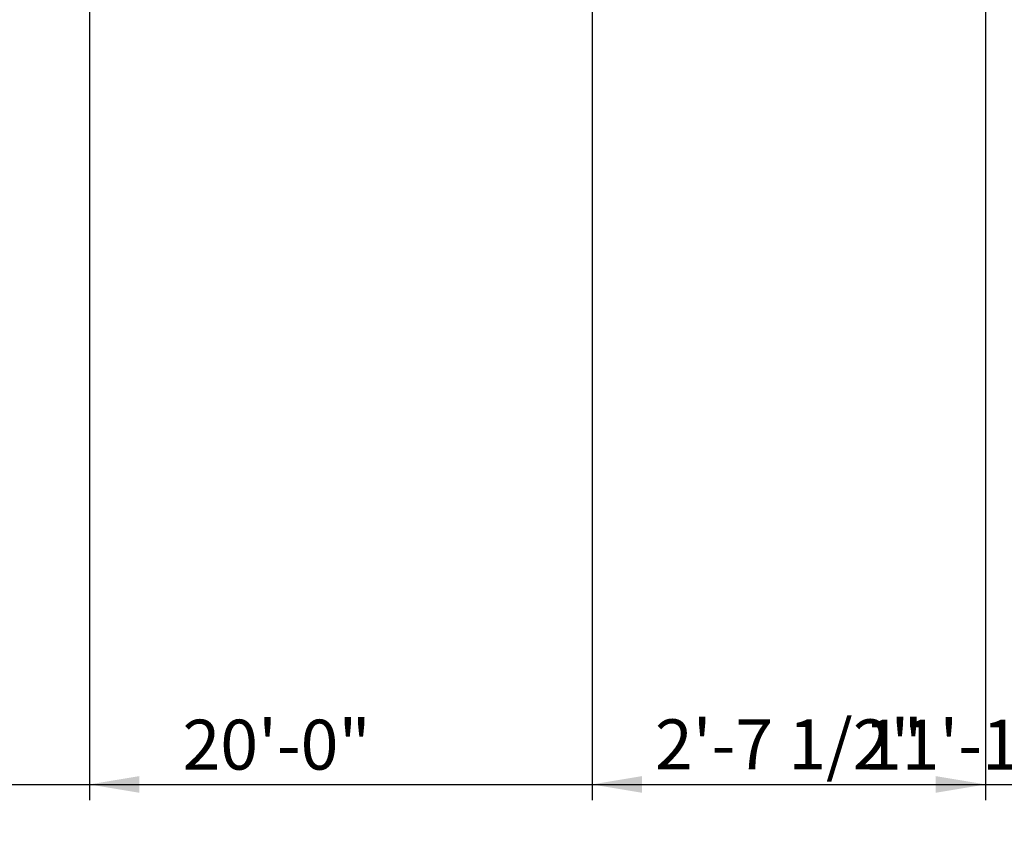
# Model space of a CAD drawing. Units: inches. Extents: x 2091 to 2899, y 967 to 2217.
# Tile 7 of 256: x 2312 to 2390, y 967 to 1032. Entities that reach past the tile are written whole.
import ezdxf

# ---------------------------------------------------------------- set-up
doc = ezdxf.new("R2010")
doc.units = ezdxf.units.IN
doc.layers.add('A-ANNO-DIMS', color=2, linetype='Continuous', lineweight=18)
doc.styles.get("Standard").update_dxf_attribs({"font": 'arial.ttf'})
doc.dimstyles.new('ISO-25', dxfattribs={"dimtxt": 4, "dimasz": 4, "dimexe": 1.25, "dimexo": 0.625, "dimtad": 1, "dimdec": 0, "dimlunit": 3, "dimtxsty": 'Standard', "dimcen": 2.5, "dimadec": 0, "dimazin": 0, "dimtfac": 1, "dimtdec": 0, "dimtmove": 0, "dimatfit": 3, "dimfxl": 1, "dimarcsym": 0})

# ---------------------------------------------------------------- blocks, each defined once
blk = doc.blocks.new('*D68')
at = {"layer": 'A-ANNO-DIMS', "color": 0, "lineweight": -2, "transparency": 16777216}
for p, q in [((2317.144, 1535.794), (2317.144, 969.464)), ((2459.384, 1535.794), (2459.384, 969.464)), ((2321.144, 970.714), (2455.384, 970.714))]:
    blk.add_line(p, q, dxfattribs=at)
at = {"layer": 'A-ANNO-DIMS', "color": 0, "transparency": 16777216}
for points in [[(2321.144, 971.381), (2321.144, 970.048), (2317.144, 970.714)], [(2455.384, 971.381), (2455.384, 970.048), (2459.384, 970.714)]]:
    blk.add_solid(points, dxfattribs=at)
at = {"layer": 'Defpoints', "color": 0, "transparency": 16777216}
for p in [(2317.144, 1536.419), (2459.384, 1536.419), (2459.384, 970.714)]:
    blk.add_point(p, dxfattribs=at)
at = {"layer": 'A-ANNO-DIMS', "color": 0, "transparency": 16777216, "insert": (2388.264, 973.382), "char_height": 4, "attachment_point": 5}
blk.add_mtext('11\'-10"', dxfattribs=at)
blk = doc.blocks.new('*D71')
at = {"layer": 'A-ANNO-DIMS', "color": 0, "lineweight": -2, "transparency": 16777216}
for p, q in [((2212.144, 1351.294), (2212.144, 969.464)), ((2452.144, 1351.294), (2452.144, 969.464)), ((2216.144, 970.714), (2448.144, 970.714))]:
    blk.add_line(p, q, dxfattribs=at)
at = {"layer": 'A-ANNO-DIMS', "color": 0, "transparency": 16777216}
for points in [[(2216.144, 971.381), (2216.144, 970.048), (2212.144, 970.714)], [(2448.144, 971.381), (2448.144, 970.048), (2452.144, 970.714)]]:
    blk.add_solid(points, dxfattribs=at)
at = {"layer": 'Defpoints', "color": 0, "transparency": 16777216}
for p in [(2212.144, 1351.919), (2452.144, 1351.919), (2452.144, 970.714)]:
    blk.add_point(p, dxfattribs=at)
at = {"layer": 'A-ANNO-DIMS', "color": 0, "transparency": 16777216, "insert": (2332.144, 973.382), "char_height": 4, "attachment_point": 5}
blk.add_mtext('20\'-0"', dxfattribs=at)
blk = doc.blocks.new('*D82')
at = {"layer": 'A-ANNO-DIMS', "color": 0, "lineweight": -2, "transparency": 16777216}
for p, q in [((2357.434, 1549.361), (2357.434, 969.464)), ((2388.969, 1549.361), (2388.969, 969.464)), ((2361.434, 970.714), (2384.969, 970.714))]:
    blk.add_line(p, q, dxfattribs=at)
at = {"layer": 'A-ANNO-DIMS', "color": 0, "transparency": 16777216}
for points in [[(2361.434, 971.381), (2361.434, 970.048), (2357.434, 970.714)], [(2384.969, 971.381), (2384.969, 970.048), (2388.969, 970.714)]]:
    blk.add_solid(points, dxfattribs=at)
at = {"layer": 'Defpoints', "color": 0, "transparency": 16777216}
for p in [(2357.434, 1549.986), (2388.969, 1549.986), (2388.969, 970.714)]:
    blk.add_point(p, dxfattribs=at)
at = {"layer": 'A-ANNO-DIMS', "color": 0, "transparency": 16777216, "insert": (2373.202, 973.408), "char_height": 4, "attachment_point": 5}
blk.add_mtext('2\'-7 1/2"', dxfattribs=at)

msp = doc.modelspace()

# ---------------------------------------------------------------- dimensions: what is measured, and where the dimension line sits
at = {"layer": 'A-ANNO-DIMS'}
for base, p1, p2, picture, middle in [((2388.969, 970.714), (2357.434, 1549.986), (2388.969, 1549.986), '*D82', (2373.202, 973.408)), ((2459.384, 970.714), (2317.144, 1536.419), (2459.384, 1536.419), '*D68', (2388.264, 973.382)), ((2452.144, 970.714), (2212.144, 1351.919), (2452.144, 1351.919), '*D71', (2332.144, 973.382))]:
    dim = msp.add_linear_dim(base=base, p1=p1, p2=p2, dimstyle='ISO-25', override={"dimdec": 1, "dimlfac": 1, "dimrnd": 0, "dimzin": 1, "dimdsep": 46, "dimlunit": 4, "dimfrac": 2}, dxfattribs=at)
    dim.commit()
    dim.dimension.update_dxf_attribs({"geometry": picture, "text_midpoint": middle})

doc.saveas('drawing.dxf')
